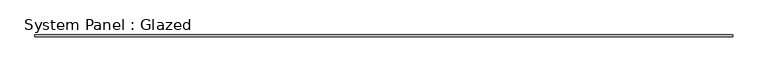
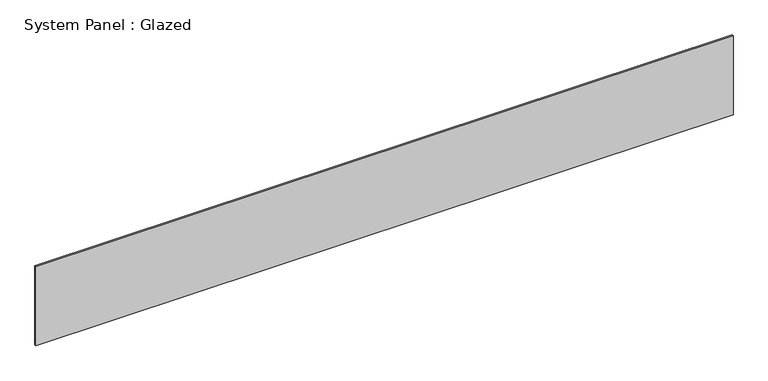
"""IFC4 building model written with IfcOpenShell, lengths in millimetres: plate geometry, System Panel : Glazed."""

from ifc_helpers import new_model, si_unit, origin, origin_with_axes, place, context, project, spatial, polyline, outline, extrude, source, transform, mapped, element, save


def system_panel_glazed_b1131520(model_context):
    return source(origin(), model_context, "Body", "SweptSolid", [
        extrude(outline(polyline([(5092.7, 19.05), (-5092.7, 19.05), (-5092.7, 44.45), (5092.7, 44.45), (5092.7, 19.05)])), origin_with_axes(), (0.0, 0.0, 1.0), 1219.2),
    ])


if __name__ == "__main__":
    model = new_model("IFC4")
    model_context = context("Model", 3, world=origin())
    ifc_project = project(units=[si_unit("LENGTHUNIT", "METRE", prefix="MILLI")], contexts=[model_context])
    site = spatial("IfcSite", under=ifc_project)
    building = spatial("IfcBuilding", under=site)
    placement = place(None, origin())
    system_panel_glazed_shape = system_panel_glazed_b1131520(model_context)
    element("IfcPlate", 1, ObjectType="System Panel : Glazed", at=placement, inside=building, context=model_context, shape_type="MappedRepresentation", body=[
        mapped(system_panel_glazed_shape, transform((0.0, 0.0, 0.0), x_axis=(1.0, 0.0, 0.0), y_axis=(0.0, 1.0, 0.0), z_axis=(0.0, 0.0, 1.0))),
    ])
    save(model, "model.ifc")

# Revit data of these elements
# Type "System Panel : Glazed"
#   Construction Type Id = "GSP4R"
#   Analytic Construction = "1/8 in Pilkington single glazing"
#   Visual Light Transmittance = 0.9
#   Solar Heat Gain Coefficient = 0.86
#   Heat Transfer Coefficient (U) = 1.18115 BTU/(h·ft²·°F)
# Element 1 (IfcPlate, "System Panel : Glazed")
#   Materials on its faces: "Glass"
# Materials
#   "Glass": class "Glass", colour RGB 0 128 192, transparency 0.75, Description = "Soda Lime Glass", Cost = 0
